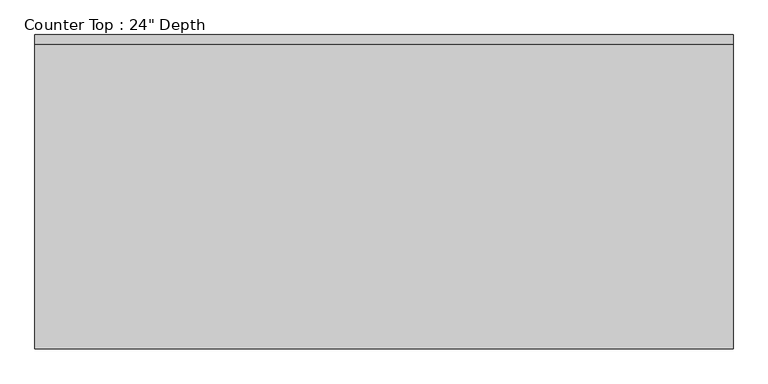
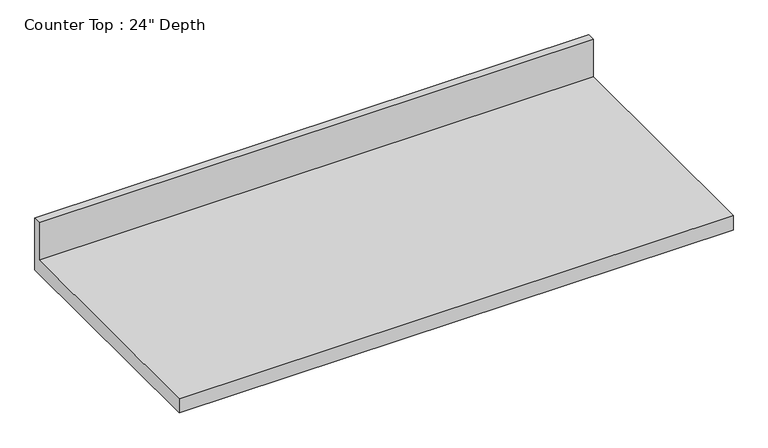
"""IFC4 building model written with IfcOpenShell, lengths in millimetres: furniture geometry."""

from ifc_helpers import new_model, si_unit, frame, origin, place, context, project, spatial, polyline, outline, extrude, source, transform, mapped, element, save


def furniture_d87d408b(model_context):
    return source(origin(), model_context, "Body", "SweptSolid", [
        extrude(outline(polyline([(0.0, 1016.0), (0.0, 876.3), (-635.0, 876.3), (-635.0, 914.4), (-19.05, 914.4), (-19.05, 1016.0), (0.0, 1016.0)])), frame((-1200.4622951, 0.0, 0.0), z_axis=(1.0, 0.0, 0.0), x_axis=(0.0, 1.0, 0.0)), (0.0, 0.0, 1.0), 1409.7),
    ])


if __name__ == "__main__":
    model = new_model("IFC4")
    model_context = context("Model", 3, world=origin())
    ifc_project = project(units=[si_unit("LENGTHUNIT", "METRE", prefix="MILLI")], contexts=[model_context])
    site = spatial("IfcSite", under=ifc_project)
    building = spatial("IfcBuilding", under=site)
    placement = place(None, origin())
    furniture_shape = furniture_d87d408b(model_context)
    element("IfcFurniture", 1, ObjectType="Counter Top : 24\" Depth", at=placement, inside=building, context=model_context, shape_type="MappedRepresentation", body=[
        mapped(furniture_shape, transform((0.0, 0.0, 0.0), x_axis=(1.0, 0.0, 0.0), y_axis=(0.0, 1.0, 0.0), z_axis=(0.0, 0.0, 1.0))),
    ])
    save(model, "model.ifc")

# Revit data of these elements
# Type "Counter Top : 24\" Depth"
#   Assembly Code = "C1030400"
#   Counter Thickness = 0' - 1 1/2"
#   Depth = 2' - 1"
#   Height = 3' - 0"
#   Length [instance default] = 8' - 0"
#   Counter Top Material = none
#   Default Elevation = 0
# Element 1 (IfcFurniture, "Counter Top : 24\" Depth")
#   Length = 4' - 7 1/2"
#   Materials on its faces: "Counter Top"
# Materials
#   "Counter Top": class "Wood", colour RGB 226 177 128, transparency 0
